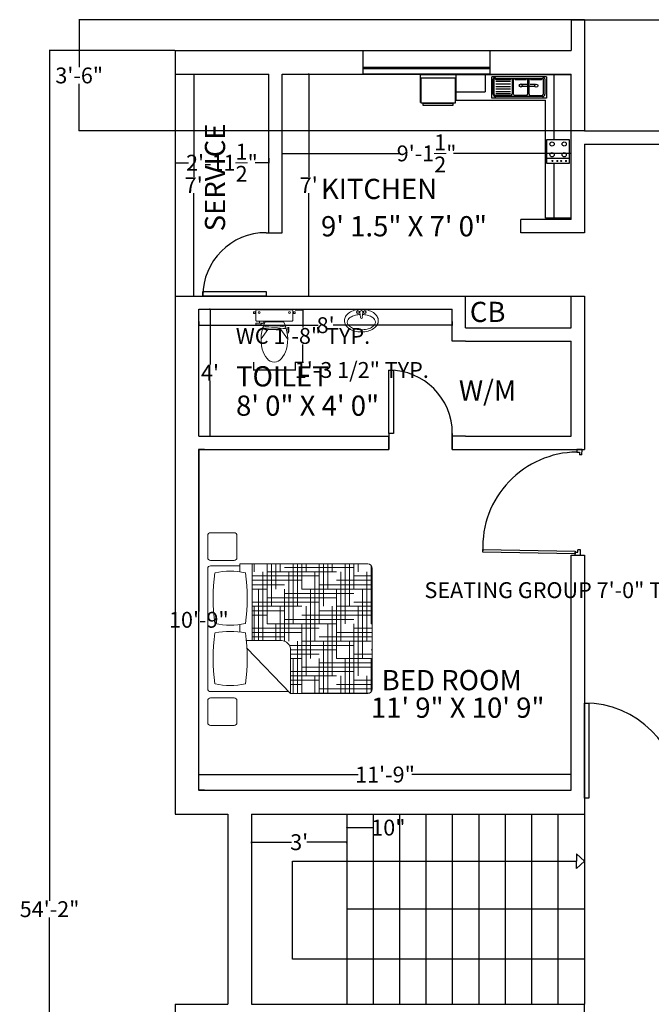
# Model space of a CAD drawing. Units: inches. Extents: x -113 to 5399, y -1393 to 3302.
# Tile 27 of 40: x 3631 to 3870, y 189 to 561. Entities that reach past the tile are written whole.
import ezdxf

# ---------------------------------------------------------------- set-up
doc = ezdxf.new("R2010")
doc.units = ezdxf.units.IN
doc.header["$MEASUREMENT"] = 0
for name, color, linetype, lineweight in [('A-ANNO-DIMS', 254, 'Continuous', 18), ('A-AREA-IDEN', 4, 'Continuous', 18), ('A-FLOR-CASE', 8, 'Continuous', 18), ('A-FLOR-FIXT', 8, 'Continuous', 18), ('doors', 2, 'Continuous', 25), ('DT TEXT', 4, 'Continuous', 18), ('furniture', 131, 'Continuous', 18), ('stairs', 210, 'Continuous', 25), ('walls', 1, 'Continuous', 25), ('windows', 3, 'Continuous', 25)]:
    doc.layers.add(name, color=color, linetype=linetype, lineweight=lineweight)
doc.layers.add('TEFRIŞ', color=11, linetype='Continuous')
doc.styles.get("Standard").update_dxf_attribs({"font": 'arial.ttf'})
doc.dimstyles.get("Standard").update_dxf_attribs({"dimtxt": 6, "dimasz": 0.18, "dimexe": 0.18, "dimexo": 0.0625, "dimgap": 0.09, "dimtad": 0, "dimtih": 1, "dimtoh": 1, "dimdec": 1, "dimzin": 0, "dimdsep": 46, "dimlunit": 4, "dimtxsty": 'Standard', "dimblk": 'ARCHTICK', "dimcen": 0.09, "dimadec": 0, "dimazin": 0, "dimtfac": 1, "dimtdec": 1, "dimtofl": 0, "dimtmove": 0, "dimatfit": 3, "dimfxl": 1, "dimtolj": 1, "dimtzin": 0, "dimarcsym": 0})

# ---------------------------------------------------------------- blocks, each defined once
blk = doc.blocks.new('*U2')
for p, q in [((0, 0), (0, -6)), ((24, 0), (24, -6))]:
    blk.add_line(p, q)
blk.add_lwpolyline([(0, 0), (0, 24), (1.75, 24), (1.75, 0)], close=True)
blk.add_arc((0, 0), 24, 0, 90)
blk = doc.blocks.new('*U3')
for p, q in [((0, 0), (0, -6)), ((36, 0), (36, -6))]:
    blk.add_line(p, q)
blk.add_lwpolyline([(0, 0), (0, 36), (1.75, 36), (1.75, 0)], close=True)
blk.add_arc((0, 0), 36, 0, 90)
blk = doc.blocks.new('*X4')
at = {"color": 0}
for p, q in [((4.359, 18.562), (4.359, 18.646)), ((4.5, 18), (4.5, 18.646)), ((4.547, 18.188), (4.547, 18.646)), ((4.594, 18.375), (4.594, 18.646)), ((4.641, 18.562), (4.641, 18.646)), ((4.781, 18), (4.781, 18.646)), ((4.828, 18.188), (4.828, 18.646)), ((4.875, 18.375), (4.875, 18.646)), ((4.922, 18.562), (4.922, 18.646)), ((5.062, 18), (5.062, 18.646)), ((5.109, 18.188), (5.109, 18.646)), ((5.156, 18.375), (5.156, 18.646)), ((5.203, 18.562), (5.203, 18.646)), ((5.344, 18), (5.344, 18.646)), ((5.391, 18.188), (5.391, 18.646)), ((5.437, 18.375), (5.437, 18.646)), ((5.484, 18.562), (5.484, 18.646)), ((5.625, 18), (5.625, 18.629)), ((4.34, 18.516), (5.062, 18.516)), ((4.453, 17.817), (4.453, 18.562)), ((4.5, 18.562), (5.25, 18.562)), ((4.687, 18.609), (5.437, 18.609)), ((4.734, 17.812), (4.734, 18.562)), ((5.016, 17.812), (5.016, 18.562)), ((5.297, 17.812), (5.297, 18.562)), ((5.437, 18.516), (5.637, 18.516)), ((5.578, 17.812), (5.578, 18.562)), ((5.625, 18.562), (5.637, 18.562)), ((4.34, 18.469), (4.875, 18.469)), ((4.34, 18.422), (4.687, 18.422)), ((5.062, 18.422), (5.637, 18.422)), ((5.25, 18.469), (5.637, 18.469)), ((4.34, 18.375), (4.5, 18.375)), ((4.406, 17.817), (4.406, 18.375)), ((4.687, 18.328), (5.437, 18.328)), ((4.687, 17.811), (4.687, 18.375)), ((4.875, 18.375), (5.625, 18.375)), ((4.969, 17.625), (4.969, 18.375)), ((5.25, 17.625), (5.25, 18.375)), ((5.531, 17.625), (5.531, 18.375)), ((4.34, 18.234), (5.062, 18.234)), ((4.5, 18.281), (5.25, 18.281)), ((5.437, 18.234), (5.637, 18.234)), ((5.625, 18.281), (5.637, 18.281)), ((4.34, 18.188), (4.875, 18.188)), ((4.34, 18.141), (4.687, 18.141)), ((4.34, 18.094), (4.5, 18.094)), ((4.359, 17.817), (4.359, 18.188)), ((4.641, 17.817), (4.641, 18.188)), ((4.875, 18.094), (5.625, 18.094)), ((4.922, 17.438), (4.922, 18.188)), ((5.062, 18.141), (5.637, 18.141)), ((5.203, 17.438), (5.203, 18.188)), ((5.25, 18.188), (5.637, 18.188)), ((5.484, 17.438), (5.484, 18.188)), ((4.5, 18), (5.25, 18)), ((4.594, 17.817), (4.594, 18)), ((4.687, 18.047), (5.437, 18.047)), ((4.875, 17.25), (4.875, 18)), ((5.156, 17.25), (5.156, 18)), ((5.437, 17.25), (5.437, 18)), ((5.625, 18), (5.637, 18)), ((4.34, 17.953), (5.062, 17.953)), ((4.34, 17.906), (4.875, 17.906)), ((5.25, 17.906), (5.637, 17.906)), ((5.437, 17.953), (5.637, 17.953)), ((4.34, 17.859), (4.687, 17.859)), ((4.828, 17.246), (4.828, 17.812)), ((4.875, 17.812), (5.625, 17.812)), ((5.062, 17.859), (5.637, 17.859)), ((5.109, 17.246), (5.109, 17.812)), ((5.391, 17.246), (5.391, 17.812)), ((4.742, 17.766), (5.437, 17.766)), ((4.755, 17.719), (5.25, 17.719)), ((4.755, 17.672), (5.062, 17.672)), ((5.437, 17.672), (5.637, 17.672)), ((5.625, 17.719), (5.637, 17.719)), ((4.755, 17.625), (4.875, 17.625)), ((4.781, 17.246), (4.781, 17.625)), ((5.062, 17.246), (5.062, 17.625)), ((5.062, 17.578), (5.637, 17.578)), ((5.25, 17.625), (5.637, 17.625)), ((5.344, 17.246), (5.344, 17.625)), ((5.625, 17.263), (5.625, 17.625)), ((4.755, 17.484), (5.437, 17.484)), ((4.875, 17.531), (5.625, 17.531)), ((4.755, 17.438), (5.25, 17.438)), ((4.755, 17.391), (5.062, 17.391)), ((4.755, 17.344), (4.875, 17.344)), ((5.016, 17.246), (5.016, 17.438)), ((5.25, 17.344), (5.637, 17.344)), ((5.297, 17.246), (5.297, 17.438)), ((5.437, 17.391), (5.637, 17.391)), ((5.578, 17.246), (5.578, 17.438)), ((5.625, 17.438), (5.637, 17.438)), ((4.875, 17.25), (5.608, 17.25)), ((4.969, 17.246), (4.969, 17.25)), ((5.062, 17.297), (5.637, 17.297)), ((5.25, 17.246), (5.25, 17.25)), ((5.531, 17.246), (5.531, 17.25))]:
    blk.add_line(p, q, dxfattribs=at)
blk = doc.blocks.new('MAT-P01')
for p, q in [((-0.021, 0.816), (-0.021, 0.56)), ((0.009, 0.846), (0.247, 0.846)), ((0.277, 0.816), (0.277, 0.56)), ((0.344, 0.816), (0.344, -0.032)), ((0.374, 0.846), (1.674, 0.846)), ((1.704, 0.816), (1.704, 0.5)), ((1.762, 0.816), (1.762, 0.56)), ((1.792, 0.846), (2.031, 0.846)), ((2.061, 0.816), (2.061, 0.56)), ((0.009, 0.53), (0.247, 0.53)), ((0.895, 0.429), (0.895, 0.049)), ((0.988, 0.5), (1.069, 0.5)), ((1.639, 0.5), (1.724, 0.5)), ((1.724, 0.5), (1.724, -0.884)), ((1.792, 0.53), (2.031, 0.53)), ((0.815, 0.423), (0.324, -0.051)), ((0.895, 0.364), (1.724, 0.364)), ((0.895, 0.364), (0.895, 0.049)), ((0.895, 0.364), (1.724, 0.364)), ((1.724, 0.364), (1.724, -0.884)), ((0.324, -0.051), (0.795, -0.051)), ((0.324, -0.051), (0.324, -0.884)), ((0.374, -0.934), (1.674, -0.934))]:
    blk.add_line(p, q)
for centre, radius, start, end in [((0.009, 0.816), 0.03, 90, 180), ((0.247, 0.816), 0.03, 0, 90), ((0.374, 0.816), 0.03, 90, 180), ((1.225, 0.603), 0.814, 168.373, 191.627), ((0.703, -1.144), 1.931, 81.8162, 98.1838), ((0.181, 0.603), 0.814, 348.373, 11.627), ((1.877, 0.603), 0.814, 168.373, 191.627), ((1.354, -1.144), 1.931, 81.8162, 98.1838), ((0.832, 0.603), 0.814, 348.373, 11.627), ((1.674, 0.816), 0.03, 0, 90), ((1.792, 0.816), 0.03, 90, 180), ((2.031, 0.816), 0.03, 0, 90), ((0.009, 0.56), 0.03, 180, 270), ((0.247, 0.56), 0.03, 270, 0), ((1.792, 0.56), 0.03, 180, 270), ((2.031, 0.56), 0.03, 270, 0), ((0.703, 2.35), 1.931, 261.8162, 278.1838), ((1.354, 2.35), 1.931, 261.8162, 278.1838), ((0.795, 0.049), 0.1, 270, 0), ((0.374, -0.884), 0.05, 180, 270), ((1.674, -0.884), 0.05, 270, 0)]:
    blk.add_arc(centre, radius, start, end)
at = {"rotation": 270}
blk.add_blockref('*X4', (-16.922, 4.704), dxfattribs=at)
blk = doc.blocks.new('A$C008029BD')
at = {"layer": 'TEFRIŞ', "ltscale": 0.05}
for p, q in [((0, 0), (0, -3.55)), ((3.37, 0), (0, 0)), ((3.37, 0), (3.37, -0.6)), ((1.522, -0.4), (0, -0.4)), ((3.37, -0.4), (2.083, -0.4)), ((0.05, -0.581), (0.05, -1.869)), ((0.05, -0.581), (0.55, -0.581)), ((0.086, -1.773), (0.086, -0.677)), ((0.096, -0.617), (0.454, -0.617)), ((0.099, -0.659), (0.457, -0.659)), ((0.514, -0.677), (0.514, -1.773)), ((0.55, -0.581), (0.55, -1.869)), ((0.6, -2.71), (0.6, -0.6)), ((3.37, -0.6), (0.6, -0.6)), ((0.113, -0.954), (0.113, -0.695)), ((0.23, -0.846), (0.229, -0.967)), ((0.28, -0.846), (0.277, -1.158)), ((0.493, -0.695), (0.493, -0.954)), ((0.096, -1.024), (0.454, -1.024)), ((0.457, -0.99), (0.099, -0.99)), ((0.11, -1.319), (0.11, -1.06)), ((0.228, -1.02), (0.227, -1.159)), ((0.49, -1.06), (0.49, -1.319)), ((0.454, -1.355), (0.096, -1.355)), ((0.096, -1.391), (0.454, -1.391)), ((0.11, -1.773), (0.11, -1.427)), ((0.154, -1.773), (0.154, -1.427)), ((0.214, -1.773), (0.214, -1.427)), ((0.274, -1.773), (0.274, -1.427)), ((0.334, -1.773), (0.334, -1.427)), ((0.39, -1.773), (0.39, -1.427)), ((0.444, -1.773), (0.444, -1.427)), ((0.49, -1.427), (0.49, -1.773)), ((0.454, -1.809), (0.096, -1.809)), ((0.454, -1.833), (0.096, -1.833)), ((0, -2.025), (0.4, -2.025)), ((0.55, -1.869), (0.05, -1.869)), ((0.4, -2.71), (0.4, -2.025)), ((0, -2.71), (0.6, -2.71)), ((0, -3.55), (0.65, -3.55))]:
    blk.add_line(p, q, dxfattribs=at)
at = {"layer": 'TEFRIŞ'}
blk.add_line((1.969, -0.05), (1.969, -0.572), dxfattribs=at)
at = {"layer": 'TEFRIŞ', "ltscale": 0.05}
for points in [[(1.522, -0.05), (2.083, -0.05), (2.083, -0.572), (1.522, -0.572)], [(0.67, -2.73), (0.67, -3.53), (0.07, -3.53), (0.07, -2.73)], [(0.72, -2.78), (0.72, -3.48), (0.67, -3.48), (0.67, -2.78)]]:
    blk.add_lwpolyline(points, close=True, dxfattribs=at)
at = {"layer": 'TEFRIŞ', "const_width": 0.025}
for points in [[(2.014, -0.123, 1), (2.039, -0.123, 1)], [(2.014, -0.236, 1), (2.039, -0.236, 1)], [(2.014, -0.327, 1), (2.039, -0.327, 1)], [(2.014, -0.44, 1), (2.039, -0.44, 1)]]:
    blk.add_lwpolyline(points, format="xyb", close=True, dxfattribs=at)
at = {"layer": 'TEFRIŞ', "ltscale": 0.05}
for centre, radius in [((1.628, -0.164), 0.0505), ((1.628, -0.45), 0.0505), ((0.255, -0.82), 0.036), ((0.252, -1.184), 0.036)]:
    blk.add_circle(centre, radius, dxfattribs=at)
at = {"layer": 'TEFRIŞ'}
for centre in [(1.88, -0.164), (1.88, -0.45)]:
    blk.add_circle(centre, 0.0505, dxfattribs=at)
at = {"layer": 'TEFRIŞ', "ltscale": 0.05}
for centre, radius, start, end in [((0.108, -0.649), 0.0351, 110.4976, 230.5777), ((0.118, -0.673), 0.023, 143.9853, 258.5157), ((0.454, -0.677), 0.06, 0, 90), ((0.457, -0.695), 0.036, 0, 90), ((0.115, -1.038), 0.023, 143.9853, 258.5157), ((0.118, -0.976), 0.023, 101.4843, 216.0147), ((0.454, -1.06), 0.036, 0, 90), ((0.457, -0.954), 0.036, 270, 0), ((0.115, -1.341), 0.023, 101.4843, 216.0147), ((0.454, -1.319), 0.036, 270, 0), ((0.115, -1.405), 0.023, 143.9853, 258.5157), ((0.454, -1.427), 0.036, 0, 90), ((0.108, -1.801), 0.0351, 129.4223, 249.5024), ((0.115, -1.796), 0.023, 101.4843, 216.0147), ((0.454, -1.773), 0.06, 270, 0), ((0.454, -1.773), 0.036, 270, 0)]:
    blk.add_arc(centre, radius, start, end, dxfattribs=at)
blk = doc.blocks.new('toilet-3')
at = {"color": 0, "linetype": 'ByBlock'}
for p, q in [((-0.281, -0.05), (-0.281, -0.069)), ((-0.281, -0.05), (-0.261, -0.05)), ((-0.281, -0.069), (-0.261, -0.069)), ((-0.261, -0.047), (-0.261, -0.072)), ((-0.261, -0.047), (-0.251, -0.047)), ((-0.261, -0.072), (-0.251, -0.072)), ((-0.251, -0.047), (-0.251, -0.072)), ((-0.25, -0.03), (-0.25, -0.165)), ((0.24, -0.02), (-0.24, -0.02)), ((0.25, -0.03), (0.25, -0.165)), ((0.261, -0.047), (0.251, -0.047)), ((0.251, -0.047), (0.251, -0.072)), ((0.261, -0.072), (0.251, -0.072)), ((0.261, -0.047), (0.261, -0.072)), ((0.281, -0.05), (0.261, -0.05)), ((0.281, -0.069), (0.261, -0.069)), ((0.281, -0.05), (0.281, -0.069)), ((-0.144, -0.2), (-0.25, -0.2)), ((-0.25, -0.2), (-0.25, -0.222)), ((-0.198, -0.222), (-0.25, -0.222)), ((0.24, -0.175), (-0.24, -0.175)), ((-0.202, -0.2), (-0.202, -0.175)), ((-0.198, -0.222), (-0.16, -0.207)), ((-0.16, -0.207), (-0.16, -0.2)), ((-0.144, -0.2), (-0.144, -0.175)), ((0.125, -0.182), (-0.125, -0.182)), ((-0.089, -0.287), (-0.18, -0.415)), ((0.089, -0.287), (-0.089, -0.287)), ((0.089, -0.287), (0.18, -0.415))]:
    blk.add_line(p, q, dxfattribs=at)
for centre in [(-0.205, -0.059), (0.205, -0.059)]:
    blk.add_circle(centre, 0.0125, dxfattribs=at)
for centre, radius, start, end in [((-0.24, -0.03), 0.01, 90, 180), ((0.24, -0.03), 0.01, 0, 90), ((-0.24, -0.165), 0.01, 180, 270), ((0.376, -0.424), 0.557, 154.2321, 193.6755), ((-0.013, -1.787), 1.521, 83.4552, 95.5271), ((-0.005, -0.896), 0.659, 75.9276, 103.0204), ((-0.376, -0.424), 0.557, 346.3245, 25.7679), ((0.24, -0.165), 0.01, 270, 0), ((0.262, -0.406), 0.452, 199.2942, 217.2549), ((-0.265, -0.4), 0.457, 322.2382, 340.1051), ((-0.001, -0.609), 0.12, 216.3794, 323.6206)]:
    blk.add_arc(centre, radius, start, end, dxfattribs=at)
blk = doc.blocks.new('wash-6')
at = {"color": 0, "linetype": 'ByBlock'}
for p, q in [((-0.036, -0.063), (-0.021, -0.18)), ((0.036, -0.063), (0.021, -0.18))]:
    blk.add_line(p, q, dxfattribs=at)
for centre, radius in [((-0.075, -0.062), 0.0325), ((-0.075, -0.062), 0.0263), ((0.075, -0.062), 0.0325), ((0.075, -0.062), 0.0263)]:
    blk.add_circle(centre, radius, dxfattribs=at)
for centre, radius, start, end in [((0, -0.56), 0.56, 90, 105.4371), ((-0.204, -0.25), 0.17, 148.1465, 180), ((-0.107, -0.311), 0.285, 123.6901, 148.1465), ((-0.114, -0.361), 0.225, 118.369, 142.5096), ((-0.042, -0.407), 0.401, 105.4371, 123.6901), ((-0.045, -0.488), 0.37, 102.6081, 118.369), ((0, -0.69), 0.576, 92.9466, 102.6081), ((0, -0.063), 0.0361, 0, 180), ((0, -0.18), 0.0215, 180, 0), ((0, -0.56), 0.56, 74.5629, 90), ((0, -0.69), 0.576, 77.3919, 87.0534), ((0.045, -0.488), 0.37, 61.631, 77.3919), ((0.042, -0.407), 0.401, 56.3099, 74.5629), ((0.114, -0.361), 0.225, 37.4904, 61.631), ((0.107, -0.311), 0.285, 31.8535, 56.3099), ((0.204, -0.25), 0.17, 0, 31.8535), ((-0.204, -0.25), 0.17, 180, 211.8535), ((-0.107, -0.189), 0.285, 211.8535, 236.3099), ((-0.217, -0.282), 0.0954, 142.5096, 180), ((-0.217, -0.282), 0.0954, 180, 217.4904), ((-0.114, -0.203), 0.225, 217.4904, 241.631), ((-0.042, -0.092), 0.401, 236.3099, 254.5629), ((-0.045, -0.076), 0.37, 241.631, 257.3919), ((0.045, -0.076), 0.37, 282.6081, 298.369), ((0.042, -0.092), 0.401, 285.4371, 303.6901), ((0.114, -0.203), 0.225, 298.369, 322.5096), ((0.107, -0.189), 0.285, 303.6901, 328.1465), ((0.217, -0.282), 0.0954, 0, 37.4904), ((0.217, -0.282), 0.0954, 322.5096, 0), ((0.204, -0.25), 0.17, 328.1465, 0), ((0, 0.06), 0.56, 254.5629, 270), ((0, 0.125), 0.576, 257.3919, 270), ((0, 0.125), 0.576, 270, 282.6081), ((0, 0.06), 0.56, 270, 285.4371)]:
    blk.add_arc(centre, radius, start, end, dxfattribs=at)
blk = doc.blocks.new('_ArchTick')
at = {"color": 0, "linetype": 'ByBlock', "const_width": 0.15}
blk.add_lwpolyline([(-0.5, -0.5), (0.5, 0.5)], dxfattribs=at)
blk = doc.blocks.new('*D92')
at = {"layer": 'A-ANNO-DIMS', "color": 0, "lineweight": -2, "transparency": 16777216}
for p, q in [((3740.54, 540.78), (3740.18, 540.78)), ((3740.36, 540.78), (3740.36, 501.87)), ((3740.36, 456.78), (3740.36, 495.69)), ((3740.54, 456.78), (3740.18, 456.78))]:
    blk.add_line(p, q, dxfattribs=at)
at = {"layer": 'Defpoints', "color": 0, "transparency": 16777216}
for p in [(3740.6, 540.78), (3740.36, 456.78), (3740.6, 456.78)]:
    blk.add_point(p, dxfattribs=at)
at = {"layer": 'A-ANNO-DIMS', "color": 0, "lineweight": -2, "transparency": 16777216, "xscale": 0.18, "yscale": 0.18, "zscale": 0.18}
for p, rotation in [((3740.36, 540.78), 90), ((3740.36, 456.78), 270)]:
    blk.add_blockref('_ArchTick', p, dxfattribs=dict(at, rotation=rotation))
at = {"layer": 'A-ANNO-DIMS', "color": 0, "transparency": 16777216, "insert": (3740.36, 498.78), "char_height": 6, "attachment_point": 5}
blk.add_mtext("\\A1;7'", dxfattribs=at)
blk = doc.blocks.new('*D93')
at = {"layer": 'A-ANNO-DIMS', "color": 0, "lineweight": -2, "transparency": 16777216}
for p, q in [((3730.23, 510.78), (3774.73, 510.78)), ((3730.23, 510.71), (3730.23, 510.6)), ((3839.73, 510.78), (3795.23, 510.78)), ((3839.73, 510.84), (3839.73, 510.96))]:
    blk.add_line(p, q, dxfattribs=at)
at = {"layer": 'Defpoints', "color": 0, "transparency": 16777216}
for p in [(3730.23, 510.78), (3839.73, 510.78), (3839.73, 510.78)]:
    blk.add_point(p, dxfattribs=at)
at = {"layer": 'A-ANNO-DIMS', "color": 0, "lineweight": -2, "transparency": 16777216, "xscale": 0.18, "yscale": 0.18, "zscale": 0.18, "rotation": 180}
blk.add_blockref('_ArchTick', (3730.23, 510.78), dxfattribs=at)
at = {"layer": 'A-ANNO-DIMS', "color": 0, "lineweight": -2, "transparency": 16777216, "xscale": 0.18, "yscale": 0.18, "zscale": 0.18}
blk.add_blockref('_ArchTick', (3839.73, 510.78), dxfattribs=at)
at = {"layer": 'A-ANNO-DIMS', "color": 0, "transparency": 16777216, "insert": (3784.98, 510.78), "char_height": 6, "attachment_point": 5}
blk.add_mtext('\\A1;9\'-1{\\H1x;\\S1/2;}"', dxfattribs=at)
blk = doc.blocks.new('*D100')
at = {"layer": 'A-ANNO-DIMS', "color": 0, "lineweight": -2, "transparency": 16777216}
for p, q in [((3689.67, 549.78), (3642.02, 549.78)), ((3642.2, 549.78), (3642.2, 227.93)), ((3642.2, -100.22), (3642.2, 221.62)), ((3689.67, -100.22), (3642.02, -100.22))]:
    blk.add_line(p, q, dxfattribs=at)
at = {"layer": 'Defpoints', "color": 0, "transparency": 16777216}
for p in [(3689.73, 549.78), (3642.2, -100.22), (3689.73, -100.22)]:
    blk.add_point(p, dxfattribs=at)
at = {"layer": 'A-ANNO-DIMS', "color": 0, "lineweight": -2, "transparency": 16777216, "xscale": 0.18, "yscale": 0.18, "zscale": 0.18}
for p, rotation in [((3642.2, 549.78), 90), ((3642.2, -100.22), 270)]:
    blk.add_blockref('_ArchTick', p, dxfattribs=dict(at, rotation=rotation))
at = {"layer": 'A-ANNO-DIMS', "color": 0, "transparency": 16777216, "insert": (3642.2, 224.78), "char_height": 6, "attachment_point": 5}
blk.add_mtext('\\A1;54\'-2"', dxfattribs=at)
blk = doc.blocks.new('*D109')
at = {"layer": 'A-ANNO-DIMS', "color": 0, "lineweight": -2, "transparency": 16777216}
for p, q in [((3718.73, 249.79), (3718.73, 250.3)), ((3718.73, 250.12), (3733.88, 250.12)), ((3754.73, 250.12), (3739.58, 250.12)), ((3754.73, 249.79), (3754.73, 250.3))]:
    blk.add_line(p, q, dxfattribs=at)
at = {"layer": 'Defpoints', "color": 0, "transparency": 16777216}
for p in [(3718.73, 249.73), (3754.73, 250.12), (3754.73, 249.73)]:
    blk.add_point(p, dxfattribs=at)
at = {"layer": 'A-ANNO-DIMS', "color": 0, "lineweight": -2, "transparency": 16777216, "xscale": 0.18, "yscale": 0.18, "zscale": 0.18, "rotation": 180}
blk.add_blockref('_ArchTick', (3718.73, 250.12), dxfattribs=at)
at = {"layer": 'A-ANNO-DIMS', "color": 0, "lineweight": -2, "transparency": 16777216, "xscale": 0.18, "yscale": 0.18, "zscale": 0.18}
blk.add_blockref('_ArchTick', (3754.73, 250.12), dxfattribs=at)
at = {"layer": 'A-ANNO-DIMS', "color": 0, "transparency": 16777216, "insert": (3736.73, 250.12), "char_height": 6, "attachment_point": 5}
blk.add_mtext("\\A1;3'", dxfattribs=at)
blk = doc.blocks.new('*D110')
at = {"layer": 'A-ANNO-DIMS', "color": 0, "lineweight": -2, "transparency": 16777216}
for p, q in [((3754.73, 255.71), (3754.73, 255.83)), ((3754.73, 255.65), (3764.73, 255.65)), ((3764.73, 255.71), (3764.73, 255.83)), ((3764.73, 255.65), (3764.91, 255.65))]:
    blk.add_line(p, q, dxfattribs=at)
at = {"layer": 'Defpoints', "color": 0, "transparency": 16777216}
for p in [(3754.73, 255.65), (3764.73, 255.65), (3764.73, 255.65)]:
    blk.add_point(p, dxfattribs=at)
at = {"layer": 'A-ANNO-DIMS', "color": 0, "lineweight": -2, "transparency": 16777216, "xscale": 0.18, "yscale": 0.18, "zscale": 0.18, "rotation": 180}
blk.add_blockref('_ArchTick', (3754.73, 255.65), dxfattribs=at)
at = {"layer": 'A-ANNO-DIMS', "color": 0, "lineweight": -2, "transparency": 16777216, "xscale": 0.18, "yscale": 0.18, "zscale": 0.18}
blk.add_blockref('_ArchTick', (3764.73, 255.65), dxfattribs=at)
at = {"layer": 'A-ANNO-DIMS', "color": 0, "transparency": 16777216, "insert": (3770.5, 255.65), "char_height": 6, "attachment_point": 5}
blk.add_mtext('\\A1;10"', dxfattribs=at)
blk = doc.blocks.new('*D111')
at = {"layer": 'A-ANNO-DIMS', "color": 0, "lineweight": -2, "transparency": 16777216}
for p, q in [((3700.82, 398.78), (3698.55, 398.78)), ((3698.73, 398.78), (3698.73, 337.43)), ((3698.73, 269.78), (3698.73, 331.12)), ((3700.82, 269.78), (3698.55, 269.78))]:
    blk.add_line(p, q, dxfattribs=at)
at = {"layer": 'Defpoints', "color": 0, "transparency": 16777216}
for p in [(3700.88, 398.78), (3698.73, 269.78), (3700.88, 269.78)]:
    blk.add_point(p, dxfattribs=at)
at = {"layer": 'A-ANNO-DIMS', "color": 0, "lineweight": -2, "transparency": 16777216, "xscale": 0.18, "yscale": 0.18, "zscale": 0.18}
for p, rotation in [((3698.73, 398.78), 90), ((3698.73, 269.78), 270)]:
    blk.add_blockref('_ArchTick', p, dxfattribs=dict(at, rotation=rotation))
at = {"layer": 'A-ANNO-DIMS', "color": 0, "transparency": 16777216, "insert": (3698.73, 334.28), "char_height": 6, "attachment_point": 5}
blk.add_mtext('\\A1;10\'-9"', dxfattribs=at)
blk = doc.blocks.new('*D112')
at = {"layer": 'A-ANNO-DIMS', "color": 0, "lineweight": -2, "transparency": 16777216}
for p, q in [((3698.73, 275.44), (3698.73, 275.89)), ((3839.73, 275.44), (3839.73, 275.89)), ((3698.73, 275.71), (3759.12, 275.71)), ((3839.73, 275.71), (3779.34, 275.71))]:
    blk.add_line(p, q, dxfattribs=at)
at = {"layer": 'Defpoints', "color": 0, "transparency": 16777216}
for p in [(3698.73, 275.71), (3698.73, 275.38), (3839.73, 275.38)]:
    blk.add_point(p, dxfattribs=at)
at = {"layer": 'A-ANNO-DIMS', "color": 0, "lineweight": -2, "transparency": 16777216, "xscale": 0.18, "yscale": 0.18, "zscale": 0.18, "rotation": 180}
blk.add_blockref('_ArchTick', (3698.73, 275.71), dxfattribs=at)
at = {"layer": 'A-ANNO-DIMS', "color": 0, "lineweight": -2, "transparency": 16777216, "xscale": 0.18, "yscale": 0.18, "zscale": 0.18}
blk.add_blockref('_ArchTick', (3839.73, 275.71), dxfattribs=at)
at = {"layer": 'A-ANNO-DIMS', "color": 0, "transparency": 16777216, "insert": (3769.23, 275.71), "char_height": 6, "attachment_point": 5}
blk.add_mtext('\\A1;11\'-9"', dxfattribs=at)
blk = doc.blocks.new('*D113')
at = {"layer": 'A-ANNO-DIMS', "color": 0, "lineweight": -2, "transparency": 16777216}
for p, q in [((3703.08, 451.78), (3702.78, 451.78)), ((3702.96, 451.78), (3702.96, 430.87)), ((3702.96, 403.78), (3702.96, 424.69)), ((3703.08, 403.78), (3702.78, 403.78))]:
    blk.add_line(p, q, dxfattribs=at)
at = {"layer": 'Defpoints', "color": 0, "transparency": 16777216}
for p in [(3703.14, 451.78), (3702.96, 403.78), (3703.14, 403.78)]:
    blk.add_point(p, dxfattribs=at)
at = {"layer": 'A-ANNO-DIMS', "color": 0, "lineweight": -2, "transparency": 16777216, "xscale": 0.18, "yscale": 0.18, "zscale": 0.18}
for p, rotation in [((3702.96, 451.78), 90), ((3702.96, 403.78), 270)]:
    blk.add_blockref('_ArchTick', p, dxfattribs=dict(at, rotation=rotation))
at = {"layer": 'A-ANNO-DIMS', "color": 0, "transparency": 16777216, "insert": (3702.96, 427.78), "char_height": 6, "attachment_point": 5}
blk.add_mtext("\\A1;4'", dxfattribs=at)
blk = doc.blocks.new('*D114')
at = {"layer": 'A-ANNO-DIMS', "color": 0, "lineweight": -2, "transparency": 16777216}
for p, q in [((3698.73, 447.11), (3698.73, 445.6)), ((3698.73, 445.78), (3743.87, 445.78)), ((3794.73, 445.78), (3749.58, 445.78)), ((3794.73, 447.11), (3794.73, 445.6))]:
    blk.add_line(p, q, dxfattribs=at)
at = {"layer": 'Defpoints', "color": 0, "transparency": 16777216}
for p in [(3698.73, 447.17), (3794.73, 447.17), (3794.73, 445.78)]:
    blk.add_point(p, dxfattribs=at)
at = {"layer": 'A-ANNO-DIMS', "color": 0, "lineweight": -2, "transparency": 16777216, "xscale": 0.18, "yscale": 0.18, "zscale": 0.18, "rotation": 180}
blk.add_blockref('_ArchTick', (3698.73, 445.78), dxfattribs=at)
at = {"layer": 'A-ANNO-DIMS', "color": 0, "lineweight": -2, "transparency": 16777216, "xscale": 0.18, "yscale": 0.18, "zscale": 0.18}
blk.add_blockref('_ArchTick', (3794.73, 445.78), dxfattribs=at)
at = {"layer": 'A-ANNO-DIMS', "color": 0, "transparency": 16777216, "insert": (3746.73, 445.78), "char_height": 6, "attachment_point": 5}
blk.add_mtext("\\A1;8'", dxfattribs=at)
blk = doc.blocks.new('*D115')
at = {"layer": 'A-ANNO-DIMS', "color": 0, "lineweight": -2, "transparency": 16777216}
for p, q in [((3689.73, 508.94), (3689.73, 507.07)), ((3689.73, 507.25), (3694.84, 507.25)), ((3725.23, 507.25), (3720.11, 507.25)), ((3725.23, 508.94), (3725.23, 507.07))]:
    blk.add_line(p, q, dxfattribs=at)
at = {"layer": 'Defpoints', "color": 0, "transparency": 16777216}
for p in [(3689.73, 509), (3725.23, 509), (3725.23, 507.25)]:
    blk.add_point(p, dxfattribs=at)
at = {"layer": 'A-ANNO-DIMS', "color": 0, "lineweight": -2, "transparency": 16777216, "xscale": 0.18, "yscale": 0.18, "zscale": 0.18, "rotation": 180}
blk.add_blockref('_ArchTick', (3689.73, 507.25), dxfattribs=at)
at = {"layer": 'A-ANNO-DIMS', "color": 0, "lineweight": -2, "transparency": 16777216, "xscale": 0.18, "yscale": 0.18, "zscale": 0.18}
blk.add_blockref('_ArchTick', (3725.23, 507.25), dxfattribs=at)
at = {"layer": 'A-ANNO-DIMS', "color": 0, "transparency": 16777216, "insert": (3707.48, 507.25), "char_height": 6, "attachment_point": 5}
blk.add_mtext('\\A1;2\'-11{\\H1x;\\S1/2;}"', dxfattribs=at)
blk = doc.blocks.new('*D116')
at = {"layer": 'A-ANNO-DIMS', "color": 0, "lineweight": -2, "transparency": 16777216}
for p, q in [((3694.84, 540.78), (3696.98, 540.78)), ((3696.8, 540.78), (3696.8, 501.87)), ((3696.8, 456.78), (3696.8, 495.69)), ((3694.84, 456.78), (3696.98, 456.78))]:
    blk.add_line(p, q, dxfattribs=at)
at = {"layer": 'Defpoints', "color": 0, "transparency": 16777216}
for p in [(3694.78, 540.78), (3694.78, 456.78), (3696.8, 456.78)]:
    blk.add_point(p, dxfattribs=at)
at = {"layer": 'A-ANNO-DIMS', "color": 0, "lineweight": -2, "transparency": 16777216, "xscale": 0.18, "yscale": 0.18, "zscale": 0.18}
for p, rotation in [((3696.8, 540.78), 90), ((3696.8, 456.78), 270)]:
    blk.add_blockref('_ArchTick', p, dxfattribs=dict(at, rotation=rotation))
at = {"layer": 'A-ANNO-DIMS', "color": 0, "transparency": 16777216, "insert": (3696.8, 498.78), "char_height": 6, "attachment_point": 5}
blk.add_mtext("\\A1;7'", dxfattribs=at)
blk = doc.blocks.new('WIN-PLAN-48IN')
h = blk.add_hatch(color=256)
h.dxf.hatch_style = 1
h.paths.add_polyline_path([(48, 2.5), (0, 2.5), (0, 2), (48, 2)])
for p, q in [((0, 9), (48, 9)), ((0, 0), (0, 9)), ((48, 9), (48, 0)), ((48, 2.5), (0, 2.5)), ((48, 2), (0, 2)), ((48, 0), (0, 0))]:
    blk.add_line(p, q)
blk = doc.blocks.new('DOOR-SINGLE-36IN-PLAN')
for p, q in [((0.5, 2), (0.5, 36.98)), ((0.5, 36.98), (1.5, 36.98)), ((1.5, 36.98), (1.5, 2)), ((0, 2), (0, 0)), ((0, 2), (1.04, 2)), ((1.5, 2), (0.5, 2)), ((1.04, 2), (1.04, 0.98)), ((1.04, 0.98), (2, 0.98)), ((2, 0), (2, 0.98)), ((38.96, 0.98), (38, 0.98)), ((38, 0), (38, 0.98)), ((40, 2), (38.96, 2)), ((38.96, 2), (38.96, 0.98)), ((40, 0), (40, 2)), ((0, 0), (2, 0)), ((0, 0), (2, 0)), ((38, 0), (40, 0))]:
    blk.add_line(p, q)
blk.add_arc((2.94, 0.99), 36.04, 1.6003, 93.0893)
blk = doc.blocks.new('*D177')
at = {"layer": 'A-ANNO-DIMS', "color": 0, "lineweight": -2, "transparency": 16777216}
for p, q in [((3735.26, 451.62), (3738.35, 451.62)), ((3738.17, 451.62), (3738.17, 444.9)), ((3738.17, 431.8), (3738.17, 438.51)), ((3735.26, 431.8), (3738.35, 431.8))]:
    blk.add_line(p, q, dxfattribs=at)
at = {"layer": 'Defpoints', "color": 0, "transparency": 16777216}
for p in [(3735.2, 451.62), (3738.17, 451.62), (3735.2, 431.8)]:
    blk.add_point(p, dxfattribs=at)
at = {"layer": 'A-ANNO-DIMS', "color": 0, "lineweight": -2, "transparency": 16777216, "xscale": 0.18, "yscale": 0.18, "zscale": 0.18}
for p, rotation in [((3738.17, 451.62), 90), ((3738.17, 431.8), 270)]:
    blk.add_blockref('_ArchTick', p, dxfattribs=dict(at, rotation=rotation))
at = {"layer": 'A-ANNO-DIMS', "color": 0, "transparency": 16777216, "insert": (3738.17, 441.71), "char_height": 6, "attachment_point": 5}
blk.add_mtext('\\A1;WC 1\'-8" TYP.', dxfattribs=at)
blk = doc.blocks.new('*D178')
at = {"layer": 'A-ANNO-DIMS', "color": 0, "lineweight": -2, "transparency": 16777216}
for p, q in [((3719.47, 431.73), (3719.47, 428.64)), ((3719.47, 428.82), (3735.2, 428.82)), ((3735.2, 431.73), (3735.2, 428.64)), ((3735.2, 428.82), (3735.38, 428.82))]:
    blk.add_line(p, q, dxfattribs=at)
at = {"layer": 'Defpoints', "color": 0, "transparency": 16777216}
for p in [(3719.47, 431.8), (3735.2, 431.8), (3735.2, 428.82)]:
    blk.add_point(p, dxfattribs=at)
at = {"layer": 'A-ANNO-DIMS', "color": 0, "lineweight": -2, "transparency": 16777216, "xscale": 0.18, "yscale": 0.18, "zscale": 0.18, "rotation": 180}
blk.add_blockref('_ArchTick', (3719.47, 428.82), dxfattribs=at)
at = {"layer": 'A-ANNO-DIMS', "color": 0, "lineweight": -2, "transparency": 16777216, "xscale": 0.18, "yscale": 0.18, "zscale": 0.18}
blk.add_blockref('_ArchTick', (3735.2, 428.82), dxfattribs=at)
at = {"layer": 'A-ANNO-DIMS', "color": 0, "transparency": 16777216, "insert": (3760.46, 428.82), "char_height": 6, "attachment_point": 5}
blk.add_mtext('\\A1;1\'-3 1/2" TYP.', dxfattribs=at)
blk = doc.blocks.new('*D185')
at = {"layer": 'A-ANNO-DIMS', "color": 0, "lineweight": -2, "transparency": 16777216}
for p, q in [((3889.72, 345.5), (3889.54, 345.5)), ((3889.72, 332.93), (3889.72, 345.68)), ((3973.94, 345.5), (3889.72, 345.5)), ((3973.94, 332.93), (3973.94, 345.68))]:
    blk.add_line(p, q, dxfattribs=at)
at = {"layer": 'Defpoints', "color": 0, "transparency": 16777216}
for p in [(3889.72, 345.5), (3889.72, 332.87), (3973.94, 332.87)]:
    blk.add_point(p, dxfattribs=at)
at = {"layer": 'A-ANNO-DIMS', "color": 0, "lineweight": -2, "transparency": 16777216, "xscale": 0.18, "yscale": 0.18, "zscale": 0.18, "rotation": 180}
blk.add_blockref('_ArchTick', (3889.72, 345.5), dxfattribs=at)
at = {"layer": 'A-ANNO-DIMS', "color": 0, "lineweight": -2, "transparency": 16777216, "xscale": 0.18, "yscale": 0.18, "zscale": 0.18}
blk.add_blockref('_ArchTick', (3973.94, 345.5), dxfattribs=at)
at = {"layer": 'A-ANNO-DIMS', "color": 0, "transparency": 16777216, "insert": (3835.08, 345.5), "char_height": 6, "attachment_point": 5}
blk.add_mtext('\\A1;SEATING GROUP 7\'-0" TYP.', dxfattribs=at)
blk = doc.blocks.new('*D210')
at = {"layer": 'A-ANNO-DIMS', "color": 0, "lineweight": -2, "transparency": 16777216}
for p, q in [((3839.79, 561.28), (4159.21, 561.28)), ((4159.03, 561.28), (4159.03, 230.43)), ((4159.03, -106.72), (4159.03, 224.12)), ((3839.79, -106.72), (4159.21, -106.72))]:
    blk.add_line(p, q, dxfattribs=at)
at = {"layer": 'Defpoints', "color": 0, "transparency": 16777216}
for p in [(3839.73, 561.28), (4159.03, 561.28), (3839.73, -106.72)]:
    blk.add_point(p, dxfattribs=at)
at = {"layer": 'A-ANNO-DIMS', "color": 0, "lineweight": -2, "transparency": 16777216, "xscale": 0.18, "yscale": 0.18, "zscale": 0.18}
for p, rotation in [((4159.03, 561.28), 90), ((4159.03, -106.72), 270)]:
    blk.add_blockref('_ArchTick', p, dxfattribs=dict(at, rotation=rotation))
at = {"layer": 'A-ANNO-DIMS', "color": 0, "transparency": 16777216, "insert": (4159.03, 227.28), "char_height": 6, "attachment_point": 5}
blk.add_mtext('\\A1;55\'-8"', dxfattribs=at)
blk = doc.blocks.new('*D211')
at = {"layer": 'A-ANNO-DIMS', "color": 0, "lineweight": -2, "transparency": 16777216}
for p, q in [((3844.67, 561.28), (3653.25, 561.28)), ((3653.43, 561.28), (3653.43, 543.43)), ((3653.43, 519.28), (3653.43, 537.12)), ((3844.67, 519.28), (3653.25, 519.28))]:
    blk.add_line(p, q, dxfattribs=at)
at = {"layer": 'Defpoints', "color": 0, "transparency": 16777216}
for p in [(3653.43, 561.28), (3844.73, 561.28), (3844.73, 519.28)]:
    blk.add_point(p, dxfattribs=at)
at = {"layer": 'A-ANNO-DIMS', "color": 0, "lineweight": -2, "transparency": 16777216, "xscale": 0.18, "yscale": 0.18, "zscale": 0.18}
for p, rotation in [((3653.43, 561.28), 90), ((3653.43, 519.28), 270)]:
    blk.add_blockref('_ArchTick', p, dxfattribs=dict(at, rotation=rotation))
at = {"layer": 'A-ANNO-DIMS', "color": 0, "transparency": 16777216, "insert": (3653.43, 540.28), "char_height": 6, "attachment_point": 5}
blk.add_mtext('\\A1;3\'-6"', dxfattribs=at)

msp = doc.modelspace()

# ---------------------------------------------------------------- linework, layer by layer
at = {"layer": 'stairs'}
for p, q in [((3754.73, 260.78), (3754.73, 188.78)), ((3764.73, 260.78), (3764.73, 188.78)), ((3774.73, 260.78), (3774.73, 188.78)), ((3784.73, 260.78), (3784.73, 188.78)), ((3794.73, 260.78), (3794.73, 188.78)), ((3804.73, 260.78), (3804.73, 188.78)), ((3814.73, 260.78), (3814.73, 188.78)), ((3824.73, 260.78), (3824.73, 188.78)), ((3834.73, 260.78), (3834.73, 188.78)), ((3844.73, 260.78), (3844.73, 188.78)), ((3734.19, 205.87), (3734.19, 242.92)), ((3734.19, 242.92), (3841.8, 242.92)), ((3844.73, 242.92), (3841.8, 245.68)), ((3841.8, 245.68), (3841.8, 242.92)), ((3844.73, 242.92), (3841.8, 240.15)), ((3841.8, 240.15), (3841.8, 242.92)), ((3844.73, 224.78), (3754.73, 224.78)), ((3844.73, 205.87), (3734.19, 205.87))]:
    msp.add_line(p, q, dxfattribs=at)
at = {"layer": 'walls'}
for p, q in [((3844.73, 561.28), (3839.73, 561.28)), ((3839.73, 561.28), (3839.73, 549.78)), ((3844.73, 561.28), (3844.73, 519.28)), ((3844.73, 561.28), (3976.73, 561.28)), ((3689.73, 549.78), (3689.73, 260.78)), ((3689.73, 549.78), (3839.73, 549.78)), ((3689.73, 540.78), (3725.23, 540.78)), ((3725.23, 480.78), (3725.23, 540.78)), ((3730.23, 480.78), (3730.23, 540.78)), ((3730.23, 540.78), (3839.73, 540.78)), ((3839.73, 485.78), (3839.73, 540.78)), ((3844.73, 519.28), (3886.73, 519.28)), ((3844.73, 514.28), (3844.73, 480.78)), ((3844.73, 514.28), (3886.73, 514.28)), ((3839.73, 485.78), (3820.73, 485.78)), ((3820.73, 480.78), (3820.73, 485.78)), ((3725.23, 480.78), (3730.23, 480.78)), ((3844.73, 480.78), (3820.73, 480.78)), ((3689.73, 456.78), (3725.23, 456.78)), ((3725.23, 456.78), (3730.23, 456.78)), ((3730.23, 456.78), (3839.73, 456.78)), ((3799.73, 444.78), (3799.73, 456.78)), ((3839.73, 444.78), (3839.73, 456.78)), ((3839.73, 456.78), (3844.73, 456.78)), ((3844.73, 456.78), (3844.73, 398.78)), ((3698.73, 403.78), (3698.73, 451.78)), ((3698.73, 451.78), (3794.73, 451.78)), ((3794.73, 439.78), (3794.73, 451.78)), ((3799.73, 444.78), (3839.73, 444.78)), ((3799.73, 439.78), (3794.73, 439.78)), ((3799.73, 439.78), (3839.73, 439.78)), ((3839.73, 403.78), (3839.73, 439.78)), ((3698.73, 403.78), (3770.73, 403.78)), ((3770.73, 398.78), (3770.73, 403.78)), ((3794.73, 398.78), (3794.73, 404.78)), ((3799.73, 403.78), (3794.73, 403.78)), ((3799.73, 403.78), (3839.73, 403.78)), ((3698.73, 269.78), (3698.73, 398.78)), ((3698.73, 398.78), (3770.73, 398.78)), ((3794.73, 398.78), (3839.73, 398.78)), ((3839.73, 398.78), (3844.73, 398.78)), ((3839.73, 269.78), (3839.73, 358.78)), ((3839.73, 358.78), (3844.73, 358.78)), ((3844.73, 358.78), (3844.73, 269.78)), ((3698.73, 269.78), (3839.73, 269.78)), ((3844.73, 269.78), (3844.73, 260.78)), ((3689.73, 260.78), (3709.73, 260.78)), ((3709.73, 260.78), (3709.73, 188.78)), ((3718.73, 260.78), (3844.73, 260.78)), ((3718.73, 260.78), (3718.73, 188.78)), ((3689.73, 188.78), (3689.73, -100.22)), ((3689.73, 188.78), (3709.73, 188.78)), ((3718.73, 188.78), (3844.73, 188.78)), ((3844.73, 179.78), (3844.73, 188.78))]:
    msp.add_line(p, q, dxfattribs=at)

# ---------------------------------------------------------------- block references
at = {"layer": 'A-FLOR-CASE', "xscale": 16.09806929200166, "yscale": 16.09806929200166, "zscale": 16.09806929200166, "rotation": 270}
msp.add_blockref('A$C008029BD', (3839.73, 540.54), dxfattribs=at)
at = {"layer": 'A-FLOR-FIXT'}
for name, p, xscale, yscale, zscale in [('toilet-3', (3727.33, 452.17), 27.95492935005888, 27.95492935005888, 27.95492935005888), ('wash-6', (3760.28, 451.78), 17.16666334294967, 17.16666334294967, 17.16666334294967)]:
    msp.add_blockref(name, p, dxfattribs=dict(at, xscale=xscale, yscale=yscale, zscale=zscale))
at = {"layer": 'doors'}
for name, p, rotation in [('*U2', (3724.23, 456.78), 90.00000000000003), ('DOOR-SINGLE-36IN-PLAN', (3843.23, 358.76), 89.09244041659038)]:
    msp.add_blockref(name, p, dxfattribs=dict(at, rotation=rotation))
for name, p in [('*U2', (3770.73, 404.78)), ('*U3', (3844.73, 266.78))]:
    msp.add_blockref(name, p, dxfattribs=at)
at = {"layer": 'doors', "xscale": -1, "rotation": 180}
msp.add_blockref('*U3', (3844.73, 182.78), dxfattribs=at)
at = {"layer": 'furniture', "xscale": 35.02364872074636, "yscale": 35.02364872074636, "zscale": 35.02364872074636, "rotation": 90}
msp.add_blockref('MAT-P01', (3731.72, 295.04), dxfattribs=at)
at = {"layer": 'windows'}
msp.add_blockref('WIN-PLAN-48IN', (3760.98, 540.78), dxfattribs=at)

# ---------------------------------------------------------------- texts
at = {"layer": 'A-AREA-IDEN'}
msp.add_text('SERVICE', height=7.647, rotation=90, dxfattribs=at).set_placement((3708.68, 481.27))
for s, height, p in [('KITCHEN', 7.647, (3745, 493.51)), ('9\' 1.5" X 7\' 0"', 7.6473, (3745, 479.39)), ('TOILET', 7.647, (3712.82, 422.58)), ('8\' 0" X 4\' 0"', 7.6473, (3712.82, 411.5)), ('BED ROOM', 7.647, (3767.97, 307.63)), ('11\' 9" X 10\' 9"', 7.6473, (3763.87, 297.21))]:
    msp.add_text(s, height=height, dxfattribs=at).set_placement(p)
at = {"layer": 'DT TEXT'}
for s, p in [('CB', (3801.35, 446.97)), (' W/M', (3794.88, 417.22))]:
    msp.add_text(s, height=7.647, dxfattribs=at).set_placement(p)

# ---------------------------------------------------------------- dimensions: what is measured, and where the dimension line sits
at = {"layer": 'A-ANNO-DIMS'}
for base, p1, p2, override, picture, middle in [((3653.43, 561.28), (3844.73, 519.28), (3844.73, 561.28), {"dimdec": 1, "dimlfac": 1, "dimrnd": 0, "dimzin": 1, "dimdsep": 46, "dimlunit": 4, "dimfrac": 2}, '*D211', (3653.43, 540.28)), ((4159.03, 561.28), (3839.73, -106.72), (3839.73, 561.28), {"dimdec": 1, "dimlfac": 1, "dimrnd": 0, "dimzin": 1, "dimdsep": 46, "dimlunit": 4, "dimfrac": 2}, '*D210', (4159.03, 227.28)), ((3642.2, -100.22), (3689.73, 549.78), (3689.73, -100.22), {"dimclrd": 0, "dimclre": 0, "dimclrt": 0}, '*D100', (3642.2, 224.78)), ((3696.8, 456.78), (3694.78, 540.78), (3694.78, 456.78), {"dimclrd": 0, "dimclre": 0, "dimclrt": 0}, '*D116', (3696.8, 498.78)), ((3702.96, 403.78), (3703.14, 451.78), (3703.14, 403.78), {"dimclrd": 0, "dimclre": 0, "dimclrt": 0}, '*D113', (3702.96, 427.78)), ((3698.73, 269.78), (3700.88, 398.78), (3700.88, 269.78), {"dimclrd": 0, "dimclre": 0, "dimclrt": 0}, '*D111', (3698.73, 334.28))]:
    dim = msp.add_linear_dim(base=base, p1=p1, p2=p2, angle=90, dimstyle='Standard', override=override, dxfattribs=at)
    dim.commit()
    dim.dimension.update_dxf_attribs({"geometry": picture, "text_midpoint": middle})
at = {"layer": 'A-ANNO-DIMS', "transparency": 33554630}
dim = msp.add_linear_dim(base=(3740.36, 456.78), p1=(3740.6, 540.78), p2=(3740.6, 456.78), angle=90, dimstyle='Standard', override={"dimclrd": 0, "dimclre": 0, "dimclrt": 0}, dxfattribs=at)
dim.commit()
dim.dimension.update_dxf_attribs({"geometry": '*D92', "text_midpoint": (3740.36, 498.78)})
dim = msp.add_linear_dim(base=(3839.73, 510.78), p1=(3730.23, 510.78), p2=(3839.73, 510.78), dimstyle='Standard', override={"dimclrd": 0, "dimclre": 0, "dimclrt": 0}, dxfattribs=at)
dim.commit()
dim.dimension.update_dxf_attribs({"geometry": '*D93', "text_midpoint": (3784.98, 510.78)})
at = {"layer": 'A-ANNO-DIMS'}
for base, p1, p2, picture, middle in [((3725.23, 507.25), (3689.73, 509), (3725.23, 509), '*D115', (3707.48, 507.25)), ((3794.73, 445.78), (3698.73, 447.17), (3794.73, 447.17), '*D114', (3746.73, 445.78)), ((3698.73, 275.71), (3839.73, 275.38), (3698.73, 275.38), '*D112', (3769.23, 275.71)), ((3764.73, 255.65), (3754.73, 255.65), (3764.73, 255.65), '*D110', (3770.5, 255.65)), ((3754.73, 250.12), (3718.73, 249.73), (3754.73, 249.73), '*D109', (3736.73, 250.12))]:
    dim = msp.add_linear_dim(base=base, p1=p1, p2=p2, dimstyle='Standard', override={"dimclrd": 0, "dimclre": 0, "dimclrt": 0}, dxfattribs=at)
    dim.commit()
    dim.dimension.update_dxf_attribs({"geometry": picture, "text_midpoint": middle})
for base, p1, p2, angle, text, picture, middle in [((3738.17, 451.62), (3735.2, 431.8), (3735.2, 451.62), 90, 'WC <> TYP.', '*D177', (3738.17, 441.71)), ((3889.72, 345.5), (3973.94, 332.87), (3889.72, 332.87), 180, 'SEATING GROUP <> TYP.', '*D185', (3835.08, 345.5))]:
    dim = msp.add_linear_dim(base=base, p1=p1, p2=p2, angle=angle, text=text, dimstyle='Standard', override={"dimdec": 1, "dimlfac": 1, "dimrnd": 0, "dimzin": 1, "dimdsep": 46, "dimlunit": 4, "dimfrac": 2}, dxfattribs=at)
    dim.commit()
    dim.dimension.update_dxf_attribs({"geometry": picture, "text_midpoint": middle})
dim = msp.add_linear_dim(base=(3735.2, 428.82), p1=(3719.47, 431.8), p2=(3735.2, 431.8), text='<> TYP.', dimstyle='Standard', override={"dimdec": 1, "dimlfac": 1, "dimrnd": 0, "dimzin": 1, "dimdsep": 46, "dimlunit": 4, "dimfrac": 2}, dxfattribs=at)
dim.commit()
dim.dimension.update_dxf_attribs({"geometry": '*D178', "text_midpoint": (3760.46, 428.82)})

doc.saveas('drawing.dxf')
